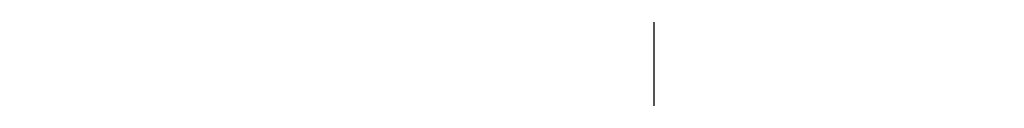
# Model space of a CAD drawing. Units: inches. Extents: x 2083 to 3317, y 1141 to 2115.
# Tile 65 of 256: x 2237.106 to 2238.294, y 1477.842 to 1477.926. Entities that reach past the tile are written whole.
import ezdxf

# ---------------------------------------------------------------- set-up
doc = ezdxf.new("R2010")
doc.units = ezdxf.units.IN
doc.layers.add('A-ANNO-DIMS', color=2, linetype='Continuous', lineweight=18)
doc.layers.add('A-WALL-PATT', color=251, linetype='Continuous', lineweight=13, true_color=0x636466)
doc.styles.get("Standard").update_dxf_attribs({"font": 'arial.ttf'})
doc.dimstyles.new('ISO-25', dxfattribs={"dimtxt": 12, "dimasz": 12, "dimexe": 1.25, "dimexo": 0.625, "dimtad": 1, "dimlunit": 3, "dimtxsty": 'Standard', "dimcen": 2.5, "dimadec": 0, "dimazin": 0, "dimtfac": 1, "dimtmove": 0, "dimatfit": 3, "dimfxl": 1, "dimarcsym": 0})

# ---------------------------------------------------------------- blocks, each defined once
blk = doc.blocks.new('*D30')
at = {"layer": 'A-ANNO-DIMS', "color": 0, "lineweight": -2, "transparency": 16777216}
for p, q in [((2240.0179, 1445.2738), (2240.0179, 1448.0455)), ((2254.3293, 1445.2738), (2254.3293, 1448.0455)), ((2228.0179, 1446.7955), (2216.0179, 1446.7955)), ((2240.0179, 1446.7955), (2254.3293, 1446.7955)), ((2266.3293, 1446.7955), (2413.7649, 1446.7955))]:
    blk.add_line(p, q, dxfattribs=at)
at = {"layer": 'A-ANNO-DIMS', "color": 0, "transparency": 16777216}
for points in [[(2228.0179, 1448.7955), (2228.0179, 1444.7955), (2240.0179, 1446.7955)], [(2266.3293, 1448.7955), (2266.3293, 1444.7955), (2254.3293, 1446.7955)]]:
    blk.add_solid(points, dxfattribs=at)
at = {"layer": 'Defpoints', "color": 0, "transparency": 16777216}
for p in [(2254.3293, 1446.7955), (2240.0179, 1444.6488), (2254.3293, 1444.6488)]:
    blk.add_point(p, dxfattribs=at)
at = {"layer": 'A-ANNO-DIMS', "color": 0, "transparency": 16777216, "insert": (2346.0471, 1453.6252), "char_height": 12, "attachment_point": 5}
blk.add_mtext('WC 1\'-2 1/2" TYP.', dxfattribs=at)
blk = doc.blocks.new('*D31')
at = {"layer": 'A-ANNO-DIMS', "color": 0, "lineweight": -2, "transparency": 16777216}
for p, q in [((2237.8711, 1456.6488), (2237.8711, 1541.9152)), ((2239.3929, 1444.6488), (2236.6211, 1444.6488)), ((2237.8711, 1431.5475), (2237.8711, 1444.6488)), ((2239.3929, 1431.5475), (2236.6211, 1431.5475)), ((2237.8711, 1419.5475), (2237.8711, 1407.5475))]:
    blk.add_line(p, q, dxfattribs=at)
at = {"layer": 'A-ANNO-DIMS', "color": 0, "transparency": 16777216}
for points in [[(2235.8711, 1456.6488), (2239.8711, 1456.6488), (2237.8711, 1444.6488)], [(2235.8711, 1419.5475), (2239.8711, 1419.5475), (2237.8711, 1431.5475)]]:
    blk.add_solid(points, dxfattribs=at)
at = {"layer": 'Defpoints', "color": 0, "transparency": 16777216}
for p in [(2237.8711, 1444.6488), (2240.0179, 1444.6488), (2240.0179, 1431.5475)]:
    blk.add_point(p, dxfattribs=at)
at = {"layer": 'A-ANNO-DIMS', "color": 0, "transparency": 16777216, "insert": (2231.2175, 1505.282), "char_height": 12, "attachment_point": 5, "rotation": 90}
blk.add_mtext('1\'-1" TYP.', dxfattribs=at)
blk = doc.blocks.new('*D45')
at = {"layer": 'A-ANNO-DIMS', "color": 0, "lineweight": -2, "transparency": 16777216}
for p, q in [((2235.9598, 1478.3864), (2235.9598, 1531.3614)), ((2418.9598, 1478.3864), (2418.9598, 1531.3614)), ((2247.9598, 1530.1114), (2406.9598, 1530.1114))]:
    blk.add_line(p, q, dxfattribs=at)
at = {"layer": 'A-ANNO-DIMS', "color": 0, "transparency": 16777216}
for points in [[(2247.9598, 1532.1114), (2247.9598, 1528.1114), (2235.9598, 1530.1114)], [(2406.9598, 1532.1114), (2406.9598, 1528.1114), (2418.9598, 1530.1114)]]:
    blk.add_solid(points, dxfattribs=at)
at = {"layer": 'Defpoints', "color": 0, "transparency": 16777216}
for p in [(2418.9598, 1530.1114), (2235.9598, 1477.7614), (2418.9598, 1477.7614)]:
    blk.add_point(p, dxfattribs=at)
at = {"layer": 'A-ANNO-DIMS', "color": 0, "transparency": 16777216, "insert": (2327.4598, 1536.8673), "char_height": 12, "attachment_point": 5}
blk.add_mtext('15\'-3"', dxfattribs=at)
blk = doc.blocks.new('*D62')
at = {"layer": 'A-ANNO-DIMS', "color": 0, "lineweight": -2, "transparency": 16777216}
for p, q in [((2235.9598, 1469.3864), (2235.9598, 1522.3614)), ((2379.9598, 1469.3864), (2379.9598, 1522.3614)), ((2247.9598, 1521.1114), (2367.9598, 1521.1114))]:
    blk.add_line(p, q, dxfattribs=at)
at = {"layer": 'A-ANNO-DIMS', "color": 0, "transparency": 16777216}
for points in [[(2247.9598, 1523.1114), (2247.9598, 1519.1114), (2235.9598, 1521.1114)], [(2367.9598, 1523.1114), (2367.9598, 1519.1114), (2379.9598, 1521.1114)]]:
    blk.add_solid(points, dxfattribs=at)
at = {"layer": 'Defpoints', "color": 0, "transparency": 16777216}
for p in [(2379.9598, 1521.1114), (2235.9598, 1468.7614), (2379.9598, 1468.7614)]:
    blk.add_point(p, dxfattribs=at)
at = {"layer": 'A-ANNO-DIMS', "color": 0, "transparency": 16777216, "insert": (2307.9598, 1527.8632), "char_height": 12, "attachment_point": 5}
blk.add_mtext('12\'-0"', dxfattribs=at)

msp = doc.modelspace()

# ---------------------------------------------------------------- hatches: boundary and pattern name
at = {"layer": 'A-WALL-PATT'}
h = msp.add_hatch(color=256, dxfattribs=at)
h.dxf.hatch_style = 1
h.paths.add_polyline_path([(3126.9598, 2020.7614), (2748.9598, 2020.7614), (2604.9598, 2020.7614), (2226.9598, 2020.7614), (2226.9598, 1702.7614), (2466.9598, 1702.7614), (2466.9598, 1582.7614), (2418.9598, 1582.7614), (2418.9598, 1477.7614), (2226.9598, 1477.7614), (2226.9598, 1263.2614), (2544.9598, 1263.2614), (2544.9598, 1411.7614), (2604.9598, 1411.7614), (2685.9598, 1411.7614), (2685.9598, 1420.7614), (2604.9598, 1420.7614), (2604.9598, 1573.7614), (2604.9598, 1702.7614), (2604.9598, 2011.7614), (2748.9598, 2011.7614), (2748.9598, 1702.7614), (2862.9598, 1702.7614), (2862.9598, 1621.7614), (2871.9598, 1621.7614), (2871.9598, 1702.7614), (2883.9598, 1702.7614), (2883.9598, 1706.9395, -0.026459), (2883.9598, 1711.7614), (2757.9598, 1711.7614), (2757.9598, 1807.7614), (2787.9598, 1807.7614), (2787.9598, 1812.2614), (2757.9598, 1812.2614), (2757.9598, 2011.7614), (2877.9598, 2011.7614), (2877.9598, 1812.2614), (2847.9598, 1812.2614), (2847.9598, 1807.7614), (2889.8357, 1807.7614), (2889.8357, 1812.2614), (2882.4598, 1812.2614), (2882.4598, 2011.7614), (3117.9598, 2011.7614), (3117.9598, 1812.2614), (2937.8357, 1812.2614), (2937.8357, 1807.7614), (2995.7098, 1807.7614), (2995.7098, 1796.1177), (3000.2098, 1796.1177), (3000.2098, 1807.7614), (3117.9598, 1807.7614), (3117.9598, 1711.7614), (3000.2098, 1711.7614), (3000.2098, 1760.1177), (2998.5727, 1760.1177, -0.020711), (2995.7098, 1760.1177), (2995.7098, 1711.7614), (2931.9598, 1711.7614), (2931.9598, 1702.7614), (3126.9598, 1702.7614)])
h.paths.add_polyline_path([(2471.4598, 2011.7614), (2471.4598, 1810.0114), (2462.7169, 1810.0114), (2462.7169, 1805.5114), (2505.9598, 1805.5114), (2505.9598, 1810.0114), (2475.9598, 1810.0114), (2475.9598, 2011.7614), (2595.9598, 2011.7614), (2595.9598, 1810.0114), (2565.9598, 1810.0114), (2565.9598, 1805.5114), (2595.9598, 1805.5114), (2595.9598, 1711.7614), (2235.9598, 1711.7614), (2235.9598, 1805.5114), (2353.7098, 1805.5114), (2353.7098, 1796.0542), (2358.2098, 1796.0542), (2358.2098, 1805.5114), (2414.7169, 1805.5114), (2414.7169, 1810.0114), (2235.9598, 1810.0114), (2235.9598, 2011.7614)], flags=16)
h.paths.add_polyline_path([(2270.2047, 1994.61), (2270.2047, 1970.61), (2246.2047, 1970.61), (2246.2047, 1994.61)], flags=0)
edge = h.paths.add_edge_path(flags=0)
edge.add_ellipse((2332.0274, 1899.7982), major_axis=(-3.043, 3.043), ratio=0.168252, start_angle=-161.3322, end_angle=-156.3071, ccw=False)
edge.add_ellipse((2333.082, 1898.7435), major_axis=(-1.0546, 1.0546), ratio=0.453532, start_angle=-123.371, end_angle=-94.1591)
edge = h.paths.add_edge_path(flags=0)
edge.add_ellipse((2332.0274, 1968.8763), major_axis=(3.043, 3.043), ratio=0.168252, start_angle=18.6678, end_angle=23.6929)
edge.add_spline(control_points=[(2332.9256, 1970.6911), (2332.2268, 1970.3361), (2330.8937, 1969.6589), (2328.4131, 1970.9321), (2327.2039, 1967.7487), (2324.7096, 1969.9556), (2322.5328, 1967.0124), (2320.0128, 1971.2958), (2317.6803, 1968.1578), (2316.0405, 1967.102), (2315.4269, 1966.8096)], knot_values=[0, 0, 0, 0, 2.267059, 4.324559, 6.685584, 8.878641, 11.121502, 14.300359, 17.755284, 19.732645, 19.732645, 19.732645, 19.732645], degree=3, periodic=0)
edge.add_ellipse((2332.0274, 1968.8763), major_axis=(3.043, 3.043), ratio=0.168252, start_angle=18.6678, end_angle=23.6929, ccw=False)
edge.add_ellipse((2333.082, 1969.9309), major_axis=(1.0546, 1.0546), ratio=0.453532, start_angle=56.629, end_angle=85.8409, ccw=False)
edge = h.paths.add_edge_path(flags=0)
edge.add_spline(control_points=[(2296.4283, 1967.9879), (2293.6278, 1965.3363), (2287.7036, 1959.7271), (2299.7439, 1949.9957), (2294.5326, 1935.6685), (2290.5732, 1920.6035), (2293.3941, 1909.9737), (2296.1854, 1904.9665)], knot_values=[0.099185, 0.099185, 0.099185, 0.099185, 0.345301, 0.619822, 0.982653, 1.386093, 1.810555, 1.810555, 1.810555, 1.810555], degree=3, periodic=0)
edge.add_spline(control_points=[(2296.1854, 1904.9665), (2297.3836, 1902.6193), (2298.001, 1901.9493), (2298.553, 1901.4682)], knot_values=[0.006246, 0.006246, 0.006246, 0.006246, 0.055476, 0.055476, 0.055476, 0.055476], degree=3, periodic=0)
edge.add_spline(control_points=[(2298.553, 1901.4682), (2297.2586, 1900.9232), (2295.2253, 1900.2321), (2293.0602, 1900.6142), (2292.1014, 1900.7884), (2292.0896, 1900.7906)], knot_values=[0.312835, 0.312835, 0.312835, 0.312835, 0.40178, 0.474987, 0.475903, 0.475903, 0.475903, 0.475903], degree=3, periodic=0)
edge.add_arc((2292.7936, 1904.6641), 3.937, 215.4209, 259.6982, ccw=False)
edge.add_spline(control_points=[(2289.5853, 1902.3823), (2289.4767, 1902.5351), (2289.3685, 1902.688), (2289.2609, 1902.8412)], knot_values=[0.102872, 0.102872, 0.102872, 0.102872, 0.116896, 0.116896, 0.116896, 0.116896], degree=3, periodic=0)
edge.add_spline(control_points=[(2289.2609, 1902.8412), (2288.6866, 1902.5502), (2287.64, 1902.0199), (2285.8813, 1901.874), (2283.853, 1901.5044), (2281.72, 1899.7105), (2278.467, 1899.4929), (2276.1571, 1901.8832), (2272.259, 1899.8041), (2267.7776, 1901.8432), (2262.2439, 1900.184), (2257.4149, 1901.7821), (2254.3184, 1900.7261), (2253.1783, 1900.3373)], knot_values=[0, 0, 0, 0, 1.907977, 3.477176, 5.261074, 7.972851, 11.680248, 13.717921, 16.939592, 22.789562, 27.502503, 33.595215, 37.145618, 37.145618, 37.145618, 37.145618], degree=3, periodic=0)
edge.add_line((2253.1783, 1900.3373), (2250.2442, 1902.8412))
edge.add_line((2250.2442, 1902.8412), (2250.2442, 1965.8333))
edge.add_line((2250.2442, 1965.8333), (2253.1783, 1968.3371))
edge.add_spline(control_points=[(2253.1783, 1968.3371), (2254.3184, 1967.9483), (2257.4149, 1966.8924), (2262.2439, 1968.4904), (2267.7776, 1966.8313), (2271.5267, 1968.5372), (2273.8759, 1967.8283), (2274.2067, 1967.7276)], knot_values=[0, 0, 0, 0, 0.09018, 0.244935, 0.364644, 0.513233, 0.537855, 0.537855, 0.537855, 0.537855], degree=3, periodic=0)
edge.add_arc((2274.3529, 1963.7933), 3.937, 72.0511, 92.1279, ccw=False)
edge.add_arc((2281.2969, 1985.23), 18.5963, 252.05113, 288.56572)
edge.add_arc((2292.3167, 1956.0289), 12.6461, 71.02679, 113.77822, ccw=False)
edge = h.paths.add_edge_path(flags=0)
edge.add_spline(control_points=[(2274.8994, 1951.8562), (2275.0662, 1951.6166), (2275.2327, 1951.3766), (2275.398, 1951.1359)], knot_values=[1.409916, 1.409916, 1.409916, 1.409916, 1.43159, 1.43159, 1.43159, 1.43159], degree=3, periodic=0)
edge.add_spline(control_points=[(2275.398, 1951.1359), (2275.7921, 1950.5619), (2276.1792, 1949.9838), (2276.5455, 1949.3971)], knot_values=[1.358238, 1.358238, 1.358238, 1.358238, 1.409916, 1.409916, 1.409916, 1.409916], degree=3, periodic=0)
edge.add_line((2276.5455, 1949.3971), (2277.4373, 1947.8622))
edge.add_spline(control_points=[(2277.4373, 1947.8622), (2276.3038, 1945.6731), (2274.6397, 1942.4269), (2274.6316, 1938.0939), (2272.7991, 1930.8515), (2274.3564, 1943.897), (2275.9477, 1947.9234), (2276.5455, 1949.3971)], knot_values=[0.005632, 0.005632, 0.005632, 0.005632, 0.186014, 0.266002, 0.357087, 0.59639, 0.739732, 0.739732, 0.739732, 0.739732], degree=3, periodic=0)
edge.add_spline(control_points=[(2276.5455, 1949.3971), (2276.1792, 1949.9838), (2275.7921, 1950.5619), (2275.398, 1951.1359)], knot_values=[1.358238, 1.358238, 1.358238, 1.358238, 1.409916, 1.409916, 1.409916, 1.409916], degree=3, periodic=0)
edge.add_spline(control_points=[(2275.398, 1951.1359), (2274.9425, 1950.0805), (2274.2078, 1948.0253), (2273.9346, 1944.8515), (2272.4685, 1937.6275), (2273.4662, 1945.6965), (2274.7006, 1951.0595), (2274.8994, 1951.8562)], knot_values=[0.104364, 0.104364, 0.104364, 0.104364, 0.189636, 0.269624, 0.36071, 0.600013, 0.644622, 0.644622, 0.644622, 0.644622], degree=3, periodic=0)
h.paths.add_polyline_path([(2269.1675, 1963.1276, -0.357527), (2268.1706, 1960.9764, -0.092561), (2268.1706, 1939.4363, -0.357527), (2269.1675, 1937.2851, -0.357527), (2267.0163, 1938.282, -0.164785), (2254.6856, 1938.282, -0.357527), (2252.5344, 1937.2851, -0.357527), (2253.5313, 1939.4363, -0.092561), (2253.5313, 1960.9764, -0.357527), (2252.5344, 1963.1276, -0.357527), (2254.6856, 1962.1307, -0.164785), (2267.0163, 1962.1307, -0.357527)], flags=0)
h.paths.add_polyline_path([(2248.8741, 1967.8018), (2248.8741, 1957.0277), (2249.4578, 1957.0277), (2249.4578, 1911.6468), (2248.8741, 1911.6468), (2248.8741, 1900.8727), (2246.5119, 1900.8727, 0.197327), (2244.1497, 1902.4569), (2244.1497, 1966.2176, 0.197327), (2246.5119, 1967.8018)], flags=0)
h.paths.add_polyline_path([(2269.1675, 1931.3893, -0.357527), (2268.1706, 1929.2381, -0.092561), (2268.1706, 1907.6981, -0.357527), (2269.1675, 1905.5469, -0.357527), (2267.0163, 1906.5438, -0.164785), (2254.6856, 1906.5438, -0.357527), (2252.5344, 1905.5469, -0.357527), (2253.5313, 1907.6981, -0.092561), (2253.5313, 1929.2381, -0.357527), (2252.5344, 1931.3893, -0.357527), (2254.6856, 1930.3925, -0.164785), (2267.0163, 1930.3925, -0.357527)], flags=0)
edge = h.paths.add_edge_path(flags=0)
edge.add_spline(control_points=[(2276.1969, 1906.7237), (2276.1681, 1909.0289), (2276.114, 1913.3719), (2270.5984, 1924.925), (2273.9052, 1919.0128), (2275.9217, 1916.2621), (2275.4746, 1912.4021), (2277.2579, 1910.3806), (2276.696, 1908.225), (2276.6462, 1906.813), (2276.6178, 1906.0084)], knot_values=[0, 0, 0, 0, 8.61026, 16.221274, 18.843057, 23.804898, 27.440828, 29.356102, 31.203478, 33.650687, 33.650687, 33.650687, 33.650687], degree=3, periodic=0)
edge.add_spline(control_points=[(2276.6178, 1906.0084), (2276.6233, 1905.6241), (2276.4977, 1904.6287), (2275.4418, 1903.8547), (2274.9373, 1903.0804), (2274.8591, 1902.8412)], knot_values=[0.156488, 0.156488, 0.156488, 0.156488, 0.184398, 0.231376, 0.250598, 0.250598, 0.250598, 0.250598], degree=3, periodic=0)
edge.add_line((2274.8591, 1902.8412), (2276.506, 1902.8412))
edge.add_spline(control_points=[(2276.506, 1902.8412), (2276.7883, 1903.0849), (2277.6651, 1904.1252), (2278.2495, 1904.3407), (2277.6539, 1908.5274), (2278.1557, 1906.2278), (2278.1005, 1905.2859), (2278.8467, 1904.069), (2277.8568, 1903.4149), (2277.8742, 1902.991), (2277.9036, 1902.8412)], knot_values=[0.059574, 0.059574, 0.059574, 0.059574, 0.080753, 0.103741, 0.16972, 0.176036, 0.207137, 0.240474, 0.262341, 0.27366, 0.27366, 0.27366, 0.27366], degree=3, periodic=0)
edge.add_line((2277.9036, 1902.8412), (2280.0298, 1902.8412))
edge.add_spline(control_points=[(2280.0298, 1902.8412), (2279.8882, 1903.0884), (2279.4993, 1903.9816), (2280.1523, 1905.9393), (2278.1036, 1909.6578), (2279.7624, 1907.1853), (2280.3279, 1904.8749), (2280.4851, 1903.4896), (2281.4633, 1903.2494), (2281.7583, 1902.9365), (2281.834, 1902.8412)], knot_values=[0.013856, 0.013856, 0.013856, 0.013856, 0.034874, 0.088867, 0.107879, 0.126738, 0.158714, 0.193757, 0.217487, 0.226722, 0.226722, 0.226722, 0.226722], degree=3, periodic=0)
edge.add_spline(control_points=[(2281.834, 1902.8412), (2281.7875, 1902.8267), (2281.647, 1902.783), (2281.3955, 1902.8595), (2281.0881, 1902.9852), (2280.7207, 1903.0609), (2280.3335, 1903.0257), (2280.1248, 1902.8989), (2280.0298, 1902.8412)], knot_values=[0, 0, 0, 0, 0.14413, 0.435517, 0.749276, 1.153046, 1.548371, 1.878348, 1.878348, 1.878348, 1.878348], degree=3, periodic=0)
edge.add_line((2280.0298, 1902.8412), (2277.9036, 1902.8412))
edge.add_spline(control_points=[(2277.9036, 1902.8412), (2277.8929, 1902.7959), (2277.8654, 1902.6796), (2277.6075, 1902.6875), (2277.2741, 1902.8007), (2276.8379, 1902.6198), (2276.5838, 1902.7893), (2276.506, 1902.8412)], knot_values=[0, 0, 0, 0, 0.127189, 0.326199, 0.628009, 1.24357, 1.515331, 1.515331, 1.515331, 1.515331], degree=3, periodic=0)
edge.add_line((2276.506, 1902.8412), (2274.8591, 1902.8412))
edge.add_spline(control_points=[(2274.8591, 1902.8412), (2274.8144, 1902.8986), (2274.7251, 1903.0134), (2274.4935, 1903.119), (2274.2443, 1902.9605), (2273.9371, 1903.1849), (2273.614, 1902.9831), (2273.4083, 1902.883), (2273.3223, 1902.8412)], knot_values=[0, 0, 0, 0, 0.21843, 0.436957, 0.687977, 0.990379, 1.398396, 1.69185, 1.69185, 1.69185, 1.69185], degree=3, periodic=0)
edge.add_spline(control_points=[(2273.3223, 1902.8412), (2273.6167, 1903.4457), (2274.274, 1904.5383), (2276.0272, 1904.5737), (2276.207, 1906.5836), (2276.1969, 1906.7237)], knot_values=[0.012227, 0.012227, 0.012227, 0.012227, 0.059472, 0.106218, 0.134458, 0.134458, 0.134458, 0.134458], degree=3, periodic=0)
h.paths.add_polyline_path([(2270.7761, 1897.7898), (2270.7761, 1873.7898), (2246.7761, 1873.7898), (2246.7761, 1897.7898)], flags=0)
h.paths.add_polyline_path([(2353.7098, 1760.0051), (2353.7098, 1760.0542), (2358.2098, 1760.0542, -0.033729)], flags=0)
h.paths.add_polyline_path([(2321.8191, 1737.5292), (2341.9953, 1737.5292, -0.414214), (2343.2033, 1736.3212), (2343.2033, 1721.0206, -0.414214), (2341.9953, 1719.8127), (2321.8191, 1719.8127, -0.414214), (2320.6112, 1721.0206), (2320.6112, 1736.3212, -0.414214)], flags=0)
h.paths.add_polyline_path([(2324.235, 1736.3212), (2339.5794, 1736.3212, -0.414214), (2341.9953, 1733.9053), (2341.9953, 1725.4497, -0.414214), (2339.5794, 1723.0338), (2333.6806, 1723.0338), (2333.8453, 1722.0455, -0.870646), (2335.4254, 1721.8259, -0.767327), (2333.9227, 1721.4232), (2331.291, 1721.4232, -0.767327), (2329.7883, 1721.8259, -0.870646), (2331.3684, 1722.0455), (2331.5331, 1723.0338), (2324.235, 1723.0338, -0.414214), (2321.8191, 1725.4497), (2321.8191, 1733.9053, -0.414214)], flags=0)
h.paths.add_polyline_path([(2570.4838, 1928.6154), (2589.6838, 1928.6154), (2590.1688, 1928.6154), (2590.1688, 1904.9934), (2570.4838, 1904.9934)], flags=0)
h.paths.add_polyline_path([(2574.4473, 1927.2638, -1), (2572.8288, 1927.2638, -1)], flags=0)
h.paths.add_polyline_path([(2573.0899, 1926.9409), (2573.925, 1927.776), (2574.1477, 1927.5533), (2573.3126, 1926.7182)], flags=0)
h.paths.add_polyline_path([(2578.7791, 1919.7296, -1), (2571.5917, 1919.7296, -1)], flags=0)
h.paths.add_polyline_path([(2578.3854, 1919.7296, -1), (2571.9854, 1919.7296, -1)], flags=0)
h.paths.add_polyline_path([(2331.5958, 1729.4762, -1), (2333.618, 1729.4762, -1)], flags=0)
h.paths.add_polyline_path([(2578.0342, 1927.2638, -1), (2576.4157, 1927.2638, -1)], flags=0)
h.paths.add_polyline_path([(2576.6889, 1927.5311), (2576.9116, 1927.7538), (2577.7467, 1926.9186), (2577.524, 1926.6959)], flags=0)
h.paths.add_polyline_path([(2578.1391, 1909.8595, -1), (2572.2317, 1909.8595, -1)], flags=0)
h.paths.add_polyline_path([(2577.7454, 1909.8595, -1), (2572.6254, 1909.8595, -1)], flags=0)
h.paths.add_polyline_path([(2583.7977, 1927.2638, -1), (2582.1792, 1927.2638, -1)], flags=0)
h.paths.add_polyline_path([(2582.7186, 1927.7538), (2583.5538, 1926.9186), (2583.3311, 1926.6959), (2582.4959, 1927.5311)], flags=0)
h.paths.add_polyline_path([(2582.4959, 1927.5311), (2582.7186, 1927.7538), (2583.5538, 1926.9186), (2583.3311, 1926.6959)], flags=0)
h.paths.add_polyline_path([(2587.7391, 1920.5296, -1), (2581.8317, 1920.5296, -1)], flags=0)
h.paths.add_polyline_path([(2587.3454, 1920.5296, -1), (2582.2254, 1920.5296, -1)], flags=0)
h.paths.add_polyline_path([(2587.3846, 1927.2638, -1), (2585.7661, 1927.2638, -1)], flags=0)
h.paths.add_polyline_path([(2586.082, 1926.9802), (2586.9172, 1927.8154), (2587.1399, 1927.5927), (2586.3047, 1926.7575)], flags=0)
h.paths.add_polyline_path([(2588.3791, 1910.6595, -1), (2581.1917, 1910.6595, -1)], flags=0)
h.paths.add_polyline_path([(2587.9854, 1910.6595, -1), (2581.5854, 1910.6595, -1)], flags=0)
h.paths.add_polyline_path([(2417.1677, 1729.4779), (2437.3439, 1729.4779, -0.414214), (2438.5519, 1728.2699), (2438.5519, 1712.9693, -0.414214), (2437.3439, 1711.7614), (2417.1677, 1711.7614, -0.414214), (2415.9598, 1712.9693), (2415.9598, 1728.2699, -0.414214)], flags=0)
h.paths.add_polyline_path([(2419.5836, 1728.2699), (2434.928, 1728.2699, -0.414214), (2437.3439, 1725.8541), (2437.3439, 1717.3984, -0.414214), (2434.928, 1714.9825), (2429.0292, 1714.9825), (2429.1939, 1713.9942, -0.870646), (2430.774, 1713.7746, -0.767327), (2429.2713, 1713.372), (2426.6396, 1713.372, -0.767327), (2425.1369, 1713.7746, -0.870646), (2426.717, 1713.9942), (2426.8817, 1714.9825), (2419.5836, 1714.9825, -0.414214), (2417.1677, 1717.3984), (2417.1677, 1725.8541, -0.414214)], flags=0)
h.paths.add_polyline_path([(2419.5836, 1728.2699), (2434.928, 1728.2699, -0.414214), (2437.3439, 1725.8541), (2437.3439, 1717.3984, -0.414214), (2434.928, 1714.9825), (2429.0292, 1714.9825), (2428.3581, 1719.009), (2427.5528, 1719.009), (2426.8817, 1714.9825), (2419.5836, 1714.9825, -0.414214), (2417.1677, 1717.3984), (2417.1677, 1725.8541, -0.414214)], flags=0)
h.paths.add_polyline_path([(2426.9444, 1721.4249, -1), (2428.9666, 1721.4249, -1)], flags=0)
h.paths.add_polyline_path([(2475.9598, 1702.7614), (2595.9598, 1702.7614), (2595.9598, 1582.7614), (2475.9598, 1582.7614)], flags=16)
h.paths.add_polyline_path([(2427.9598, 1573.7614), (2595.9598, 1573.7614), (2595.9598, 1468.7614), (2595.9598, 1420.7614), (2384.4598, 1420.7614), (2384.4598, 1468.7614), (2427.9598, 1468.7614)], flags=16)
h.paths.add_polyline_path([(2379.9598, 1468.7614), (2379.9598, 1420.7614), (2235.9598, 1420.7614), (2235.9598, 1468.7614)], flags=16)
h.paths.add_polyline_path([(2317.816, 1466.6958), (2337.9922, 1466.6958, -0.414214), (2339.2002, 1465.4878), (2339.2002, 1450.1872, -0.414214), (2337.9922, 1448.9792), (2317.816, 1448.9792, -0.414214), (2316.6081, 1450.1872), (2316.6081, 1465.4878, -0.414214)], flags=0)
h.paths.add_polyline_path([(2320.2319, 1465.4878), (2335.5763, 1465.4878, -0.414214), (2337.9922, 1463.0719), (2337.9922, 1454.6163, -0.414214), (2335.5763, 1452.2004), (2329.6775, 1452.2004), (2329.8422, 1451.212, -0.870646), (2331.4223, 1450.9925, -0.767327), (2329.9196, 1450.5898), (2327.2879, 1450.5898, -0.767327), (2325.7852, 1450.9925, -0.870646), (2327.3653, 1451.212), (2327.53, 1452.2004), (2320.2319, 1452.2004, -0.414214), (2317.816, 1454.6163), (2317.816, 1463.0719, -0.414214)], flags=0)
h.paths.add_polyline_path([(2320.2319, 1465.4878), (2335.5763, 1465.4878, -0.414214), (2337.9922, 1463.0719), (2337.9922, 1454.6163, -0.414214), (2335.5763, 1452.2004), (2329.6775, 1452.2004), (2329.0064, 1456.2269), (2328.2011, 1456.2269), (2327.53, 1452.2004), (2320.2319, 1452.2004, -0.414214), (2317.816, 1454.6163), (2317.816, 1463.0719, -0.414214)], flags=0)
h.paths.add_polyline_path([(2327.5926, 1458.6428, -1), (2329.6148, 1458.6428, -1)], flags=0)
h.paths.add_polyline_path([(2244.4117, 1433.3405), (2241.9209, 1433.3405, -0.414214), (2240.0179, 1435.2435), (2240.0179, 1440.9528, -0.414211), (2241.9209, 1442.8559), (2244.4117, 1442.8559, -1.976472)], flags=0)
h.paths.add_polyline_path([(2245.3569, 1434.3975, -0.414214), (2245.3569, 1441.7988, -2.144098)], flags=0)
h.paths.add_polyline_path([(2535.9598, 1416.2614), (2535.9598, 1272.2614), (2235.9598, 1272.2614), (2235.9598, 1416.2614)], flags=16)
h.paths.add_polyline_path([(2260.1196, 1384.2928), (2260.1196, 1362.0386), (2237.8654, 1362.0386), (2237.8654, 1384.2928)], flags=0)
edge = h.paths.add_edge_path(flags=0)
edge.add_line((2318.2518, 1362.0933), (2318.1458, 1362.001))
edge.add_ellipse((2317.4451, 1360.431), major_axis=(2.8216, 2.8216), ratio=0.168252, start_angle=18.6678, end_angle=20.9481, ccw=False)
edge.add_ellipse((2318.423, 1361.409), major_axis=(0.9779, 0.9779), ratio=0.453532, start_angle=56.629, end_angle=70.2262, ccw=False)
edge = h.paths.add_edge_path(flags=0)
edge.add_line((2319.1074, 1295.5711), (2319.015, 1295.6771))
edge.add_ellipse((2317.4451, 1296.3778), major_axis=(-2.8216, 2.8216), ratio=0.168252, start_angle=-161.3322, end_angle=-159.0519, ccw=False)
edge.add_ellipse((2318.423, 1295.3999), major_axis=(-0.9779, 0.9779), ratio=0.453532, start_angle=-123.371, end_angle=-109.7738)
edge = h.paths.add_edge_path(flags=0)
edge.add_spline(control_points=[(2284.2103, 1301.1702), (2284.5807, 1300.4447), (2284.8912, 1299.892), (2285.1596, 1299.461)], knot_values=[0.039066, 0.039066, 0.039066, 0.039066, 0.055476, 0.055476, 0.055476, 0.055476], degree=3, periodic=0)
edge.add_line((2285.1596, 1299.461), (2284.2103, 1301.1702))
edge = h.paths.add_edge_path(flags=0)
edge.add_line((2280.4125, 1297.298), (2283.37, 1297.0361))
edge.add_line((2283.37, 1297.0361), (2286.4057, 1297.9263))
edge.add_spline(control_points=[(2286.4057, 1297.9263), (2285.3055, 1297.4631), (2284.3448, 1297.1292), (2283.37, 1297.0361)], knot_values=[0.394369, 0.394369, 0.394369, 0.394369, 0.475903, 0.475903, 0.475903, 0.475903], degree=3, periodic=0)
edge.add_spline(control_points=[(2283.37, 1297.0361), (2283.2814, 1297.0277), (2282.3163, 1296.9573), (2281.3125, 1297.1345), (2280.4234, 1297.296), (2280.4125, 1297.298)], knot_values=[0.312835, 0.312835, 0.312835, 0.312835, 0.320246, 0.393453, 0.394369, 0.394369, 0.394369, 0.394369], degree=3, periodic=0)
edge = h.paths.add_edge_path(flags=0)
edge.add_line((2284.4356, 1359.6073), (2280.4463, 1355.328))
edge.add_line((2280.4463, 1355.328), (2279.58, 1351.0178))
edge.add_line((2279.58, 1351.0178), (2282.413, 1346.5804))
edge.add_spline(control_points=[(2282.413, 1346.5804), (2283.1533, 1345.5892), (2284.2529, 1344.0289), (2284.801, 1342.3872), (2284.9352, 1341.8055)], knot_values=[1.240098, 1.240098, 1.240098, 1.240098, 1.332892, 1.382712, 1.382712, 1.382712, 1.382712], degree=3, periodic=0)
edge.add_spline(control_points=[(2284.9352, 1341.8055), (2285.3191, 1340.1406), (2285.233, 1338.4092), (2284.9099, 1336.6541)], knot_values=[1.097484, 1.097484, 1.097484, 1.097484, 1.240098, 1.240098, 1.240098, 1.240098], degree=3, periodic=0)
edge.add_spline(control_points=[(2284.9099, 1336.6541), (2284.5868, 1334.899), (2284.0267, 1333.1203), (2283.4626, 1331.3606)], knot_values=[0.95487, 0.95487, 0.95487, 0.95487, 1.097484, 1.097484, 1.097484, 1.097484], degree=3, periodic=0)
edge.add_line((2283.4626, 1331.3606), (2281.8904, 1326.1534))
edge.add_line((2281.8904, 1326.1534), (2280.7563, 1321.0561))
edge.add_line((2280.7563, 1321.0561), (2280.2992, 1316.002))
edge.add_line((2280.2992, 1316.002), (2280.7159, 1310.9501))
edge.add_line((2280.7159, 1310.9501), (2282.0281, 1305.9721))
edge.add_line((2282.0281, 1305.9721), (2284.2103, 1301.1702))
edge.add_spline(control_points=[(2284.2103, 1301.1702), (2283.3407, 1302.7302), (2282.6119, 1304.3365), (2282.0281, 1305.9721)], knot_values=[0.099185, 0.099185, 0.099185, 0.099185, 0.241799, 0.241799, 0.241799, 0.241799], degree=3, periodic=0)
edge.add_spline(control_points=[(2282.0281, 1305.9721), (2281.4443, 1307.6078), (2281.0055, 1309.2728), (2280.7159, 1310.9501)], knot_values=[0.241799, 0.241799, 0.241799, 0.241799, 0.384413, 0.384413, 0.384413, 0.384413], degree=3, periodic=0)
edge.add_spline(control_points=[(2280.7159, 1310.9501), (2280.4332, 1312.5876), (2280.2894, 1314.277), (2280.2989, 1315.962), (2280.2992, 1316.002)], knot_values=[0.384413, 0.384413, 0.384413, 0.384413, 0.523647, 0.527028, 0.527028, 0.527028, 0.527028], degree=3, periodic=0)
edge.add_spline(control_points=[(2280.2992, 1316.002), (2280.3123, 1317.687), (2280.4779, 1319.3679), (2280.7563, 1321.0561)], knot_values=[0.527028, 0.527028, 0.527028, 0.527028, 0.669642, 0.669642, 0.669642, 0.669642], degree=3, periodic=0)
edge.add_spline(control_points=[(2280.7563, 1321.0561), (2281.0346, 1322.7443), (2281.4259, 1324.4396), (2281.8904, 1326.1534)], knot_values=[0.669642, 0.669642, 0.669642, 0.669642, 0.812256, 0.812256, 0.812256, 0.812256], degree=3, periodic=0)
edge.add_spline(control_points=[(2281.8904, 1326.1534), (2282.2644, 1327.5333), (2282.7879, 1329.2618), (2283.3528, 1331.0178), (2283.4626, 1331.3606)], knot_values=[0.812256, 0.812256, 0.812256, 0.812256, 0.927087, 0.95487, 0.95487, 0.95487, 0.95487], degree=3, periodic=0)
edge.add_line((2283.4626, 1331.3606), (2284.9099, 1336.6541))
edge.add_line((2284.9099, 1336.6541), (2284.9352, 1341.8055))
edge.add_line((2284.9352, 1341.8055), (2282.413, 1346.5804))
edge.add_spline(control_points=[(2282.413, 1346.5804), (2281.2751, 1348.1038), (2280.0784, 1349.5703), (2279.58, 1351.0178)], knot_values=[1.382712, 1.382712, 1.382712, 1.382712, 1.525326, 1.525326, 1.525326, 1.525326], degree=3, periodic=0)
edge.add_spline(control_points=[(2279.58, 1351.0178), (2279.4433, 1351.4147), (2279.1363, 1352.8569), (2279.7352, 1354.2904), (2280.4463, 1355.328)], knot_values=[1.525326, 1.525326, 1.525326, 1.525326, 1.564439, 1.667941, 1.667941, 1.667941, 1.667941], degree=3, periodic=0)
edge.add_spline(control_points=[(2280.4463, 1355.328), (2281.4261, 1356.7578), (2282.9308, 1358.1826), (2284.4356, 1359.6073)], knot_values=[1.667941, 1.667941, 1.667941, 1.667941, 1.810555, 1.810555, 1.810555, 1.810555], degree=3, periodic=0)
edge.add_arc((2280.6231, 1348.5182), 11.7262, 71.02679, 113.77822)
edge.add_arc((2270.4049, 1375.5952), 17.2436, 252.05113, 288.56572, ccw=False)
edge.add_arc((2263.966, 1355.7178), 3.6506, 72.0511, 92.1279)
edge.add_arc((2263.966, 1355.7178), 3.6506, 92.1279, 177.9851)
edge.add_spline(control_points=[(2260.3176, 1355.8462), (2260.2604, 1354.2207), (2260.5513, 1350.1865), (2262.9993, 1346.7663), (2264.4727, 1344.649)], knot_values=[1.43159, 1.43159, 1.43159, 1.43159, 1.564144, 1.770695, 1.770695, 1.770695, 1.770695], degree=3, periodic=0)
edge.add_line((2264.4727, 1344.649), (2264.9356, 1343.9825))
edge.add_spline(control_points=[(2263.801, 1340.2481), (2263.8432, 1340.5141), (2264.0672, 1341.7565), (2264.5127, 1343.0025), (2264.935, 1343.9811)], knot_values=[0.53657, 0.53657, 0.53657, 0.53657, 0.559349, 0.644622, 0.644622, 0.644622, 0.644622], degree=3, periodic=0)
edge.add_spline(control_points=[(2264.935, 1343.9811), (2265.1178, 1343.715), (2265.2989, 1343.4479), (2265.4768, 1343.1794)], knot_values=[1.384077, 1.384077, 1.384077, 1.384077, 1.409916, 1.409916, 1.409916, 1.409916], degree=3, periodic=0)
edge.add_spline(control_points=[(2265.4768, 1343.1794), (2265.6546, 1342.9108), (2265.8293, 1342.6408), (2265.9991, 1342.3688)], knot_values=[1.358238, 1.358238, 1.358238, 1.358238, 1.384077, 1.384077, 1.384077, 1.384077], degree=3, periodic=0)
edge.add_line((2265.9991, 1342.3688), (2266.826, 1340.9455))
edge.add_spline(control_points=[(2266.826, 1340.9455), (2268.8944, 1337.0897), (2271.3982, 1325.843), (2270.5162, 1310.5686), (2275.9194, 1301.8606), (2277.7895, 1299.1994)], knot_values=[0.116896, 0.116896, 0.116896, 0.116896, 0.472987, 1.050969, 1.313793, 1.313793, 1.313793, 1.313793], degree=3, periodic=0)
edge.add_spline(control_points=[(2277.7895, 1299.1994), (2277.8394, 1299.1285), (2277.8894, 1299.0575), (2277.9396, 1298.9866)], knot_values=[0.109884, 0.109884, 0.109884, 0.109884, 0.116896, 0.116896, 0.116896, 0.116896], degree=3, periodic=0)
edge.add_line((2277.9396, 1298.9866), (2277.7888, 1299.1991))
edge.add_spline(control_points=[(2277.7888, 1299.1991), (2277.2566, 1298.9294), (2276.2864, 1298.4379), (2275.0394, 1298.3344), (2274.3833, 1298.2389), (2274.2153, 1298.2093)], knot_values=[33.12187, 33.12187, 33.12187, 33.12187, 35.029056, 36.598255, 37.144827, 37.144827, 37.144827, 37.144827], degree=3, periodic=0)
edge.add_line((2274.2153, 1298.2093), (2273.0731, 1297.893))
edge.add_spline(control_points=[(2273.0731, 1297.893), (2272.3229, 1297.5798), (2271.0392, 1296.5105), (2269.2484, 1296.2261), (2268.4231, 1296.3747)], knot_values=[26.532584, 26.532584, 26.532584, 26.532584, 29.198919, 31.839101, 31.839101, 31.839101, 31.839101], degree=3, periodic=0)
edge.add_line((2268.4231, 1296.3747), (2263.8785, 1297.4575))
edge.add_spline(control_points=[(2263.8785, 1297.4575), (2263.5561, 1297.3594), (2261.8603, 1296.8387), (2260.2388, 1297.2824), (2258.9335, 1297.5165)], knot_values=[15.919551, 15.919551, 15.919551, 15.919551, 16.939592, 21.226067, 21.226067, 21.226067, 21.226067], degree=3, periodic=0)
edge.add_line((2258.9335, 1297.5165), (2254.0552, 1297.329))
edge.add_spline(control_points=[(2254.0552, 1297.329), (2253.7555, 1297.2958), (2252.1137, 1297.1652), (2250.4619, 1297.5442), (2249.1297, 1297.6679)], knot_values=[5.306517, 5.306517, 5.306517, 5.306517, 6.276435, 10.613034, 10.613034, 10.613034, 10.613034], degree=3, periodic=0)
edge.add_line((2249.1297, 1297.6679), (2244.3316, 1296.8778))
edge.add_line((2244.3316, 1296.8778), (2241.611, 1299.1994))
edge.add_line((2241.611, 1299.1994), (2241.611, 1357.6094))
edge.add_line((2241.611, 1357.6094), (2244.3316, 1359.9311))
edge.add_line((2244.3316, 1359.9311), (2252.7288, 1359.5427))
edge.add_spline(control_points=[(2252.7288, 1359.5427), (2252.8709, 1359.5464), (2253.3057, 1359.5482), (2253.7398, 1359.5143), (2254.0317, 1359.4824)], knot_values=[0.233291, 0.233291, 0.233291, 0.233291, 0.244935, 0.268927, 0.268927, 0.268927, 0.268927], degree=3, periodic=0)
edge.add_line((2254.0317, 1359.4824), (2259.5872, 1359.4164))
edge.add_spline(control_points=[(2259.5872, 1359.4164), (2260.6771, 1359.6285), (2262.0732, 1359.897), (2263.5237, 1359.4593), (2263.8304, 1359.366)], knot_values=[0.422516, 0.422516, 0.422516, 0.422516, 0.513233, 0.537855, 0.537855, 0.537855, 0.537855], degree=3, periodic=0)
edge.add_arc((2263.966, 1355.7178), 3.6506, 72.0511, 92.1279, ccw=False)
edge.add_arc((2270.4049, 1375.5952), 17.2436, 252.05113, 288.56572)
edge.add_arc((2280.6231, 1348.5182), 11.7262, 71.02679, 113.77822, ccw=False)
h.paths.add_polyline_path([(2240.3405, 1359.4347), (2240.3405, 1349.4444), (2240.8818, 1349.4444), (2240.8818, 1307.3645), (2240.3405, 1307.3645), (2240.3405, 1297.3741), (2238.1502, 1297.3741, 0.197327), (2235.9598, 1298.8431), (2235.9598, 1357.9657, 0.197327), (2238.1502, 1359.4347)], flags=0)
h.paths.add_polyline_path([(2259.1578, 1355.1005, -0.357527), (2258.2334, 1353.1058, -0.092561), (2258.2334, 1333.1326, -0.357527), (2259.1578, 1331.1379, -0.357527), (2257.1631, 1332.0622, -0.164785), (2245.7293, 1332.0622, -0.357527), (2243.7346, 1331.1379, -0.357527), (2244.6589, 1333.1326, -0.092561), (2244.6589, 1353.1058, -0.357527), (2243.7346, 1355.1005, -0.357527), (2245.7293, 1354.1761, -0.164785), (2257.1631, 1354.1761, -0.357527)], flags=0)
edge = h.paths.add_edge_path(flags=0)
edge.add_line((2265.9991, 1342.3688), (2266.826, 1340.9455))
edge.add_line((2266.826, 1340.9455), (2265.3076, 1337.8141))
edge.add_line((2265.3076, 1337.8141), (2264.3582, 1334.6529))
edge.add_line((2264.3582, 1334.6529), (2264.262, 1333.7997))
edge.add_spline(control_points=[(2264.262, 1333.7997), (2264.2084, 1333.1871), (2264.1621, 1332.3655), (2264.0071, 1331.4139), (2263.969, 1331.2018)], knot_values=[0.464444, 0.464444, 0.464444, 0.464444, 0.516691, 0.531608, 0.531608, 0.531608, 0.531608], degree=3, periodic=0)
edge.add_spline(control_points=[(2263.969, 1331.2018), (2263.7745, 1330.1189), (2263.4244, 1328.7908), (2263.2574, 1328.5307), (2263.234, 1328.5146)], knot_values=[0.372682, 0.372682, 0.372682, 0.372682, 0.44885, 0.464444, 0.464444, 0.464444, 0.464444], degree=3, periodic=0)
edge.add_spline(control_points=[(2263.234, 1328.5146), (2263.0964, 1328.4202), (2263.1312, 1329.3015), (2263.275, 1330.6157)], knot_values=[0.280919, 0.280919, 0.280919, 0.280919, 0.372682, 0.372682, 0.372682, 0.372682], degree=3, periodic=0)
edge.add_spline(control_points=[(2263.275, 1330.6157), (2263.4187, 1331.93), (2263.6715, 1333.6773), (2263.9699, 1335.315)], knot_values=[0.189157, 0.189157, 0.189157, 0.189157, 0.280919, 0.280919, 0.280919, 0.280919], degree=3, periodic=0)
edge.add_spline(control_points=[(2263.9699, 1335.315), (2264.1005, 1336.0322), (2264.4188, 1337.6219), (2264.7548, 1338.8644), (2264.9474, 1339.4911)], knot_values=[0.097394, 0.097394, 0.097394, 0.097394, 0.137578, 0.189157, 0.189157, 0.189157, 0.189157], degree=3, periodic=0)
edge.add_spline(control_points=[(2264.9474, 1339.4911), (2265.29, 1340.6061), (2265.6442, 1341.494), (2265.9991, 1342.3688)], knot_values=[0.005632, 0.005632, 0.005632, 0.005632, 0.097394, 0.097394, 0.097394, 0.097394], degree=3, periodic=0)
h.paths.add_polyline_path([(2259.1578, 1325.671, -0.357527), (2258.2334, 1323.6763, -0.092561), (2258.2334, 1303.7031, -0.357527), (2259.1578, 1301.7084, -0.357527), (2257.1631, 1302.6327, -0.164785), (2245.7293, 1302.6327, -0.357527), (2243.7346, 1301.7084, -0.357527), (2244.6589, 1303.7031, -0.092561), (2244.6589, 1323.6763, -0.357527), (2243.7346, 1325.671, -0.357527), (2245.7293, 1324.7466, -0.164785), (2257.1631, 1324.7466, -0.357527)], flags=0)
edge = h.paths.add_edge_path(flags=0)
edge.add_spline(control_points=[(2261.7089, 1317.3114), (2261.6795, 1317.4176), (2261.7619, 1317.3885), (2262.4907, 1316.0899), (2262.9622, 1315.3009)], knot_values=[14.955861, 14.955861, 14.955861, 14.955861, 16.221274, 18.694826, 18.694826, 18.694826, 18.694826], degree=3, periodic=0)
edge.add_spline(control_points=[(2262.9622, 1315.3009), (2262.9904, 1315.2536), (2263.7021, 1314.0674), (2264.349, 1313.1272), (2264.7301, 1312.1642)], knot_values=[18.694826, 18.694826, 18.694826, 18.694826, 18.843057, 22.433791, 22.433791, 22.433791, 22.433791], degree=3, periodic=0)
edge.add_spline(control_points=[(2264.7301, 1312.1642), (2264.8756, 1311.7964), (2265.1769, 1310.7698), (2265.1431, 1309.5593), (2265.2477, 1308.8242)], knot_values=[22.433791, 22.433791, 22.433791, 22.433791, 23.804898, 26.172756, 26.172756, 26.172756, 26.172756], degree=3, periodic=0)
edge.add_line((2265.2477, 1308.8242), (2265.8508, 1307.1719))
edge.add_spline(control_points=[(2265.8508, 1307.1719), (2266.065, 1306.8217), (2266.3844, 1306.3322), (2266.4244, 1305.7805), (2266.4204, 1305.6112)], knot_values=[28.062562, 28.062562, 28.062562, 28.062562, 29.356102, 29.911721, 29.911721, 29.911721, 29.911721], degree=3, periodic=0)
edge.add_spline(control_points=[(2266.4204, 1305.6112), (2266.4161, 1305.4326), (2266.394, 1305.25), (2266.3648, 1305.0659)], knot_values=[29.911721, 29.911721, 29.911721, 29.911721, 30.497837, 30.497837, 30.497837, 30.497837], degree=3, periodic=0)
edge.add_line((2266.3648, 1305.0659), (2266.0662, 1302.1363))
edge.add_spline(control_points=[(2266.0662, 1302.1363), (2266.0712, 1301.78), (2265.9981, 1301.2), (2265.6633, 1300.759), (2265.5089, 1300.5859)], knot_values=[0.156488, 0.156488, 0.156488, 0.156488, 0.184398, 0.203543, 0.203543, 0.203543, 0.203543], degree=3, periodic=0)
edge.add_line((2265.5089, 1300.5859), (2264.4353, 1299.1994))
edge.add_line((2264.4353, 1299.1994), (2265.9624, 1299.1994))
edge.add_line((2265.9624, 1299.1994), (2267.336, 1301.1753))
edge.add_line((2267.336, 1301.1753), (2267.3117, 1301.9862))
edge.add_spline(control_points=[(2267.3117, 1301.9862), (2267.2611, 1302.8624), (2267.1602, 1303.7371), (2267.2715, 1303.3259)], knot_values=[0.126229, 0.126229, 0.126229, 0.126229, 0.166617, 0.166617, 0.166617, 0.166617], degree=3, periodic=0)
edge.add_spline(control_points=[(2267.2715, 1303.3259), (2267.28, 1303.2943), (2267.3098, 1303.1754), (2267.3735, 1302.8836), (2267.4061, 1302.6828), (2267.4179, 1302.601)], knot_values=[0.166617, 0.166617, 0.166617, 0.166617, 0.16972, 0.176036, 0.180765, 0.180765, 0.180765, 0.180765], degree=3, periodic=0)
edge.add_spline(control_points=[(2267.7439, 1300.9875), (2267.6876, 1301.1509), (2267.4805, 1301.6567), (2267.4838, 1302.1448), (2267.4179, 1302.601)], knot_values=[0.180765, 0.180765, 0.180765, 0.180765, 0.193767, 0.220139, 0.220139, 0.220139, 0.220139], degree=3, periodic=0)
edge.add_line((2267.4179, 1302.601), (2267.7439, 1300.9875))
edge.add_spline(control_points=[(2267.7439, 1300.9875), (2267.832, 1300.7319), (2267.932, 1300.3099), (2267.5548, 1299.9745), (2267.4294, 1299.8292)], knot_values=[0.220139, 0.220139, 0.220139, 0.220139, 0.240474, 0.25489, 0.25489, 0.25489, 0.25489], degree=3, periodic=0)
edge.add_line((2267.4294, 1299.8292), (2267.2584, 1299.1994))
edge.add_line((2267.2584, 1299.1994), (2269.23, 1299.1994))
edge.add_spline(control_points=[(2269.23, 1299.1994), (2269.0987, 1299.4287), (2268.8428, 1300.0163), (2269.0116, 1300.9159), (2268.9468, 1301.6607)], knot_values=[0.013856, 0.013856, 0.013856, 0.013856, 0.034874, 0.067073, 0.067073, 0.067073, 0.067073], degree=3, periodic=0)
edge.add_line((2268.9468, 1301.6607), (2268.4316, 1303.6031))
edge.add_spline(control_points=[(2268.4316, 1303.6031), (2268.1756, 1304.1924), (2267.5962, 1305.2513), (2268.0407, 1304.6232), (2268.2514, 1304.2824)], knot_values=[0.090155, 0.090155, 0.090155, 0.090155, 0.107879, 0.120289, 0.120289, 0.120289, 0.120289], degree=3, periodic=0)
edge.add_spline(control_points=[(2268.2514, 1304.2824), (2268.3609, 1304.1053), (2269.0578, 1302.918), (2269.3827, 1301.5904), (2269.5214, 1300.7759), (2269.5752, 1300.5558)], knot_values=[0.120289, 0.120289, 0.120289, 0.120289, 0.126738, 0.158714, 0.173506, 0.173506, 0.173506, 0.173506], degree=3, periodic=0)
edge.add_line((2269.5752, 1300.5558), (2270.6858, 1299.4213))
edge.add_spline(control_points=[(2270.6858, 1299.4213), (2270.7672, 1299.3573), (2270.8379, 1299.2814), (2270.9029, 1299.1994)], knot_values=[0.21816, 0.21816, 0.21816, 0.21816, 0.226722, 0.226722, 0.226722, 0.226722], degree=3, periodic=0)
edge.add_line((2270.9372, 1299.1929), (2270.9029, 1299.1994))
edge.add_spline(control_points=[(2270.9029, 1299.1994), (2270.8598, 1299.186), (2270.7295, 1299.1455), (2270.4963, 1299.2164), (2270.2717, 1299.3083), (2270.121, 1299.348), (2270.0633, 1299.3596)], knot_values=[0.939174, 0.939174, 0.939174, 0.939174, 1.083304, 1.374691, 1.68845, 1.878348, 1.878348, 1.878348, 1.878348], degree=3, periodic=0)
edge.add_line((2270.0633, 1299.3596), (2269.23, 1299.1994))
edge.add_line((2269.23, 1299.1994), (2267.2584, 1299.1994))
edge.add_spline(control_points=[(2267.2584, 1299.1994), (2267.2484, 1299.1574), (2267.223, 1299.0497), (2266.9838, 1299.0569), (2266.8092, 1299.1162), (2266.6769, 1299.1091), (2266.6365, 1299.1048)], knot_values=[0.757665, 0.757665, 0.757665, 0.757665, 0.884854, 1.083864, 1.385675, 1.515331, 1.515331, 1.515331, 1.515331], degree=3, periodic=0)
edge.add_spline(control_points=[(2266.6365, 1299.1048), (2266.4852, 1299.0888), (2266.2358, 1299.0171), (2266.0346, 1299.1513), (2265.9624, 1299.1994)], knot_values=[0, 0, 0, 0, 0.485905, 0.757665, 0.757665, 0.757665, 0.757665], degree=3, periodic=0)
edge.add_line((2265.9624, 1299.1994), (2264.4353, 1299.1994))
edge.add_line((2264.4353, 1299.1994), (2263.8584, 1299.3671))
edge.add_spline(control_points=[(2263.8584, 1299.3671), (2263.8189, 1299.3709), (2263.7795, 1299.3857), (2263.7401, 1299.4015)], knot_values=[0.845925, 0.845925, 0.845925, 0.845925, 0.978627, 0.978627, 0.978627, 0.978627], degree=3, periodic=0)
edge.add_line((2263.7218, 1299.3964), (2263.0103, 1299.1994))
edge.add_spline(control_points=[(2263.0103, 1299.1994), (2263.2458, 1299.6829), (2263.506, 1300.1281), (2263.8735, 1300.408)], knot_values=[0.012227, 0.012227, 0.012227, 0.012227, 0.052971, 0.052971, 0.052971, 0.052971], degree=3, periodic=0)
edge.add_spline(control_points=[(2263.8735, 1300.408), (2263.9321, 1300.4527), (2264.0842, 1300.553), (2264.2552, 1300.6242), (2264.3597, 1300.6647)], knot_values=[0.052971, 0.052971, 0.052971, 0.052971, 0.059472, 0.069086, 0.069086, 0.069086, 0.069086], degree=3, periodic=0)
edge.add_line((2264.3597, 1300.6647), (2265.1419, 1301.0778))
edge.add_line((2265.1419, 1301.0778), (2265.6758, 1302.7996))
edge.add_line((2265.6758, 1302.7996), (2265.5407, 1305.7041))
edge.add_line((2265.5407, 1305.7041), (2264.8031, 1309.3277))
edge.add_line((2264.8031, 1309.3277), (2263.0405, 1314.0918))
edge.add_spline(control_points=[(2263.0405, 1314.0918), (2262.3836, 1315.6714), (2261.796, 1316.9977), (2261.7089, 1317.3114)], knot_values=[11.216896, 11.216896, 11.216896, 11.216896, 14.955861, 14.955861, 14.955861, 14.955861], degree=3, periodic=0)
h.paths.add_polyline_path([(2871.9598, 1416.2614), (2895.91, 1416.2614), (2895.91, 1420.7614), (2871.9598, 1420.7614), (2871.9598, 1501.7614), (2862.9598, 1501.7614), (2862.9598, 1420.7614), (2805.9598, 1420.7614), (2805.9598, 1411.7614), (2862.9598, 1411.7614), (2862.9598, 1263.2614), (3126.9598, 1263.2614), (3126.9598, 1411.7614), (3126.9598, 1486.7614), (2943.9598, 1486.7614), (2943.9598, 1477.7614), (2967.8603, 1477.7614), (2967.8603, 1420.7614), (2943.91, 1420.7614), (2943.91, 1416.2614), (3117.9598, 1416.2614), (3117.9598, 1420.7614), (2972.3603, 1420.7614), (2972.3603, 1477.7614), (3117.9598, 1477.7614), (3117.9598, 1420.7614), (3117.9598, 1272.2614), (2871.9598, 1272.2614)], flags=0)
h.paths.add_polyline_path([(2457.1256, 1485.9425), (2527.6027, 1485.9425), (2527.6027, 1537.6357), (2457.1256, 1537.6357)], flags=8)
h.paths.add_polyline_path([(2481.0051, 1609.9818), (2590.7658, 1609.9818), (2590.7658, 1682.0034), (2481.0051, 1682.0034)], flags=8)
h.paths.add_polyline_path([(2483.085, 1729.1268), (2553.562, 1729.1268), (2553.562, 1780.82), (2483.085, 1780.82)], flags=8)

# ---------------------------------------------------------------- dimensions: what is measured, and where the dimension line sits
at = {"layer": 'A-ANNO-DIMS'}
for base, p1, p2, picture, middle in [((2418.9598, 1530.1114), (2235.9598, 1477.7614), (2418.9598, 1477.7614), '*D45', (2327.4598, 1536.8673)), ((2379.9598, 1521.1114), (2235.9598, 1468.7614), (2379.9598, 1468.7614), '*D62', (2307.9598, 1527.8632))]:
    dim = msp.add_linear_dim(base=base, p1=p1, p2=p2, dimstyle='ISO-25', override={"dimdec": 1, "dimlfac": 1, "dimrnd": 0, "dimzin": 1, "dimdsep": 46, "dimlunit": 4, "dimfrac": 2}, dxfattribs=at)
    dim.commit()
    dim.dimension.update_dxf_attribs({"geometry": picture, "text_midpoint": middle})
dim = msp.add_linear_dim(base=(2237.8711, 1444.6488), p1=(2240.0179, 1431.5475), p2=(2240.0179, 1444.6488), angle=90, text='<> TYP.', dimstyle='ISO-25', override={"dimdec": 1, "dimlfac": 1, "dimrnd": 0, "dimzin": 1, "dimdsep": 46, "dimlunit": 4, "dimfrac": 2}, dxfattribs=at)
dim.commit()
dim.dimension.update_dxf_attribs({"geometry": '*D31', "text_midpoint": (2231.2175, 1505.282)})
dim = msp.add_linear_dim(base=(2254.3293, 1446.7955), p1=(2240.0179, 1444.6488), p2=(2254.3293, 1444.6488), text='WC <> TYP.', dimstyle='ISO-25', override={"dimdec": 1, "dimlfac": 1, "dimrnd": 0, "dimzin": 1, "dimdsep": 46, "dimlunit": 4, "dimfrac": 2}, dxfattribs=at)
dim.commit()
dim.dimension.update_dxf_attribs({"geometry": '*D30', "text_midpoint": (2346.0471, 1453.6252)})

doc.saveas('drawing.dxf')
